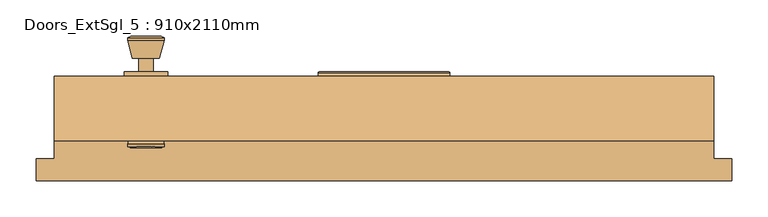
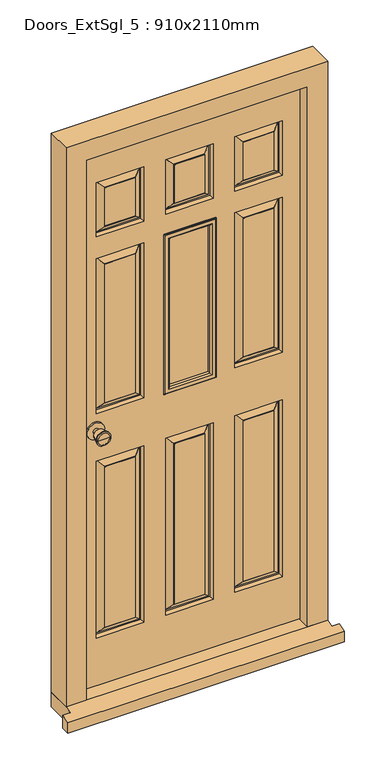
"""IFC4 building model written with IfcOpenShell, lengths in millimetres: door geometry, Doors_ExtSgl_5 : 910x2110mm."""

from ifc_helpers import new_model, si_unit, point, frame, frame_2d, origin, place, context, project, spatial, polyline, circle_curve, ellipse_curve, trimmed, segment, composite_curve, outline, extrude, faceted_brep, source, transform, mapped, element, save
from ifc_brep_helpers import plane_surface, cylinder_surface, revolved_surface, advanced_brep


def doors_extsgl_5_910x2110mm_99758a98(model_context):
    return source(origin(), model_context, "Body", "SolidModel", [
        advanced_brep(
        [(-328.4666667, 18.4, 1000.0), (-338.4666667, 18.4, 1000.0), (-318.4666667, 18.4, 1000.0), (-307.9907991, 67.4, 1000.0), (-348.9425342, 67.4, 1000.0), (-328.4666667, 67.4, 1000.0), (-303.4666667, 65.5721319, 1000.0), (-353.4666667, 65.5721319, 1000.0), (-303.4666667, 62.1084537, 1000.0), (-353.4666667, 62.1084537, 1000.0), (-309.8304306, 37.4, 1000.0), (-347.1029027, 37.4, 1000.0), (-318.4666667, 37.4, 1000.0), (-338.4666667, 37.4, 1000.0)],
        [
            (0, 1),
            (1, 2, circle_curve(frame((-328.4666667, 18.4, 1000.0), z_axis=(0.0, -1.0, 0.0), x_axis=(-1.0, 0.0, 0.0)), 10.0)),
            (2, 0),
            (2, 1, circle_curve(frame((-328.4666667, 18.4, 1000.0), z_axis=(0.0, -1.0, 0.0), x_axis=(-1.0, 0.0, 0.0)), 10.0)),
            (3, 4, circle_curve(frame((-328.4666667, 67.4, 1000.0), z_axis=(0.0, 1.0, 0.0), x_axis=(-1.0, 0.0, 0.0)), 20.4758676)),
            (4, 5),
            (5, 3),
            (4, 3, circle_curve(frame((-328.4666667, 67.4, 1000.0), z_axis=(0.0, 1.0, 0.0), x_axis=(-1.0, 0.0, 0.0)), 20.4758676)),
            (6, 7, circle_curve(frame((-328.4666667, 65.5721319, 1000.0), z_axis=(0.0, 1.0, 0.0), x_axis=(-1.0, 0.0, 0.0)), 25.0)),
            (7, 4),
            (3, 6),
            (7, 6, circle_curve(frame((-328.4666667, 65.5721319, 1000.0), z_axis=(0.0, 1.0, 0.0), x_axis=(-1.0, 0.0, 0.0)), 25.0)),
            (8, 9, circle_curve(frame((-328.4666667, 62.1084537, 1000.0), z_axis=(0.0, 1.0, 0.0), x_axis=(-1.0, 0.0, 0.0)), 25.0)),
            (9, 7),
            (6, 8),
            (9, 8, circle_curve(frame((-328.4666667, 62.1084537, 1000.0), z_axis=(0.0, 1.0, 0.0), x_axis=(-1.0, 0.0, 0.0)), 25.0)),
            (10, 11, circle_curve(frame((-328.4666667, 37.4, 1000.0), z_axis=(0.0, 1.0, 0.0), x_axis=(-1.0, 0.0, 0.0)), 18.636236)),
            (11, 9),
            (8, 10),
            (11, 10, circle_curve(frame((-328.4666667, 37.4, 1000.0), z_axis=(0.0, 1.0, 0.0), x_axis=(-1.0, 0.0, 0.0)), 18.636236)),
            (12, 13, circle_curve(frame((-328.4666667, 37.4, 1000.0), z_axis=(0.0, 1.0, 0.0), x_axis=(-1.0, 0.0, 0.0)), 10.0)),
            (13, 11),
            (10, 12),
            (13, 12, circle_curve(frame((-328.4666667, 37.4, 1000.0), z_axis=(0.0, 1.0, 0.0), x_axis=(-1.0, 0.0, 0.0)), 10.0)),
            (1, 13),
            (12, 2),
        ],
        [
            plane_surface(frame((-328.4666667, 18.4, 1000.0), z_axis=(0.0, -1.0, 0.0), x_axis=(-1.0, 0.0, 0.0))),
            plane_surface(frame((-328.4666667, 67.4, 1000.0), z_axis=(0.0, 1.0, 0.0), x_axis=(-1.0, 0.0, 0.0))),
            revolved_surface(polyline([(-348.9425342, 67.4, 1000.0), (-353.4666667, 65.5721319, 1000.0)]), (-328.4666667, 18.4, 1000.0), (0.0, -1.0, 0.0)),
            cylinder_surface(frame((-328.4666667, 18.4, 1000.0), z_axis=(0.0, -1.0, 0.0), x_axis=(-1.0, 0.0, 0.0)), 25.0),
            revolved_surface(polyline([(-353.4666667, 62.1084537, 1000.0), (-347.1029027, 37.4, 1000.0)]), (-328.4666667, 18.4, 1000.0), (0.0, -1.0, 0.0)),
            plane_surface(frame((-328.4666667, 37.4, 1000.0), z_axis=(0.0, -1.0, 0.0), x_axis=(-1.0, 0.0, 0.0))),
            cylinder_surface(frame((-328.4666667, 18.4, 1000.0), z_axis=(0.0, -1.0, 0.0), x_axis=(-1.0, 0.0, 0.0)), 10.0),
        ],
        [
            (0, [[1, 2, 3]]),
            (0, [[-3, 4, -1]]),
            (1, [[5, 6, 7]]),
            (1, [[8, -7, -6]]),
            (2, [[9, 10, -5, 11]]),
            (2, [[12, -11, -8, -10]]),
            (3, [[13, 14, -9, 15]]),
            (3, [[16, -15, -12, -14]]),
            (4, [[17, 18, -13, 19]]),
            (4, [[20, -19, -16, -18]]),
            (5, [[21, 22, -17, 23]]),
            (5, [[24, -23, -20, -22]]),
            (6, [[-2, 25, -21, 26]]),
            (6, [[-4, -26, -24, -25]]),
        ],
    ),
        extrude(outline(composite_curve([segment(trimmed(circle_curve(frame_2d((1000.0, -328.4666667)), 30.0), [point((1000.0, -358.4666667))], [point((1000.0, -298.4666667))], False, "CARTESIAN"), True, "CONTINUOUS"), segment(trimmed(circle_curve(frame_2d((1000.0, -328.4666667)), 30.0), [point((1000.0, -298.4666667))], [point((1000.0, -358.4666667))], False, "CARTESIAN"), True, "CONTINUOUS")], self_intersect=False)), frame((0.0, 12.4, 0.0), z_axis=(0.0, 1.0, 0.0), x_axis=(0.0, 0.0, 1.0)), (0.0, 0.0, 1.0), 6.0),
        advanced_brep(
        [(-328.4666667, -37.6, 1000.0), (-318.4666667, -37.6, 1000.0), (-338.4666667, -37.6, 1000.0), (-307.9907991, -86.6, 1000.0), (-328.4666667, -86.6, 1000.0), (-348.9425342, -86.6, 1000.0), (-303.4666667, -84.7721319, 1000.0), (-353.4666667, -84.7721319, 1000.0), (-303.4666667, -81.3084537, 1000.0), (-353.4666667, -81.3084537, 1000.0), (-309.8304306, -56.6, 1000.0), (-347.1029027, -56.6, 1000.0), (-318.4666667, -56.6, 1000.0), (-338.4666667, -56.6, 1000.0)],
        [
            (0, 1),
            (1, 2, circle_curve(frame((-328.4666667, -37.6, 1000.0), z_axis=(0.0, 1.0, 0.0), x_axis=(-1.0, 0.0, 0.0)), 10.0)),
            (2, 0),
            (2, 1, circle_curve(frame((-328.4666667, -37.6, 1000.0), z_axis=(0.0, 1.0, 0.0), x_axis=(-1.0, 0.0, 0.0)), 10.0)),
            (3, 4),
            (4, 5),
            (5, 3, circle_curve(frame((-328.4666667, -86.6, 1000.0), z_axis=(0.0, -1.0, 0.0), x_axis=(-1.0, 0.0, 0.0)), 20.4758676)),
            (3, 5, circle_curve(frame((-328.4666667, -86.6, 1000.0), z_axis=(0.0, -1.0, 0.0), x_axis=(-1.0, 0.0, 0.0)), 20.4758676)),
            (6, 3),
            (5, 7),
            (7, 6, circle_curve(frame((-328.4666667, -84.7721319, 1000.0), z_axis=(0.0, -1.0, 0.0), x_axis=(-1.0, 0.0, 0.0)), 25.0)),
            (6, 7, circle_curve(frame((-328.4666667, -84.7721319, 1000.0), z_axis=(0.0, -1.0, 0.0), x_axis=(-1.0, 0.0, 0.0)), 25.0)),
            (8, 6),
            (7, 9),
            (9, 8, circle_curve(frame((-328.4666667, -81.3084537, 1000.0), z_axis=(0.0, -1.0, 0.0), x_axis=(-1.0, 0.0, 0.0)), 25.0)),
            (8, 9, circle_curve(frame((-328.4666667, -81.3084537, 1000.0), z_axis=(0.0, -1.0, 0.0), x_axis=(-1.0, 0.0, 0.0)), 25.0)),
            (10, 8),
            (9, 11),
            (11, 10, circle_curve(frame((-328.4666667, -56.6, 1000.0), z_axis=(0.0, -1.0, 0.0), x_axis=(-1.0, 0.0, 0.0)), 18.636236)),
            (10, 11, circle_curve(frame((-328.4666667, -56.6, 1000.0), z_axis=(0.0, -1.0, 0.0), x_axis=(-1.0, 0.0, 0.0)), 18.636236)),
            (12, 10),
            (11, 13),
            (13, 12, circle_curve(frame((-328.4666667, -56.6, 1000.0), z_axis=(0.0, -1.0, 0.0), x_axis=(-1.0, 0.0, 0.0)), 10.0)),
            (12, 13, circle_curve(frame((-328.4666667, -56.6, 1000.0), z_axis=(0.0, -1.0, 0.0), x_axis=(-1.0, 0.0, 0.0)), 10.0)),
            (1, 12),
            (13, 2),
        ],
        [
            plane_surface(frame((-328.4666667, -37.6, 1000.0), z_axis=(0.0, 1.0, 0.0), x_axis=(-1.0, 0.0, 0.0))),
            plane_surface(frame((-328.4666667, -86.6, 1000.0), z_axis=(0.0, -1.0, 0.0), x_axis=(-1.0, 0.0, 0.0))),
            revolved_surface(polyline([(-348.9425342, -86.6, 1000.0), (-353.4666667, -84.7721319, 1000.0)]), (-328.4666667, -37.6, 1000.0), (0.0, 1.0, 0.0)),
            cylinder_surface(frame((-328.4666667, -37.6, 1000.0), z_axis=(0.0, 1.0, 0.0), x_axis=(-1.0, 0.0, 0.0)), 25.0),
            revolved_surface(polyline([(-353.4666667, -81.3084537, 1000.0), (-347.1029027, -56.6, 1000.0)]), (-328.4666667, -37.6, 1000.0), (0.0, 1.0, 0.0)),
            plane_surface(frame((-328.4666667, -56.6, 1000.0), z_axis=(0.0, 1.0, 0.0), x_axis=(-1.0, 0.0, 0.0))),
            cylinder_surface(frame((-328.4666667, -37.6, 1000.0), z_axis=(0.0, 1.0, 0.0), x_axis=(-1.0, 0.0, 0.0)), 10.0),
        ],
        [
            (0, [[1, 2, 3]]),
            (0, [[-3, 4, -1]]),
            (1, [[5, 6, 7]]),
            (1, [[-6, -5, 8]]),
            (2, [[9, -7, 10, 11]]),
            (2, [[-10, -8, -9, 12]]),
            (3, [[13, -11, 14, 15]]),
            (3, [[-14, -12, -13, 16]]),
            (4, [[17, -15, 18, 19]]),
            (4, [[-18, -16, -17, 20]]),
            (5, [[21, -19, 22, 23]]),
            (5, [[-22, -20, -21, 24]]),
            (6, [[25, -23, 26, -2]]),
            (6, [[-26, -24, -25, -4]]),
        ],
    ),
        extrude(outline(composite_curve([segment(trimmed(circle_curve(frame_2d((1000.0, -328.4666667)), 30.0), [point((1000.0, -358.4666667))], [point((1000.0, -298.4666667))], False, "CARTESIAN"), True, "CONTINUOUS"), segment(trimmed(circle_curve(frame_2d((1000.0, -328.4666667)), 30.0), [point((1000.0, -298.4666667))], [point((1000.0, -358.4666667))], False, "CARTESIAN"), True, "CONTINUOUS")], self_intersect=False)), frame((0.0, -37.6, 0.0), z_axis=(0.0, 1.0, 0.0), x_axis=(0.0, 0.0, 1.0)), (0.0, 0.0, 1.0), 6.0),
        faceted_brep([(384.5333333, -76.6, 54.5), (384.5333333, -34.6, 54.5), (406.5333333, -34.6, 54.5), (406.5333333, 12.4, 54.5), (455.0333333, 12.4, 54.5), (455.0333333, -76.6, 54.5), (455.0333333, -76.6, 2110.0), (-454.9666667, -76.6, 2110.0), (-454.9666667, -76.6, 54.5), (-384.4666667, -76.6, 54.5), (-384.4666667, -76.6, 2039.5), (384.5333333, -76.6, 2039.5), (455.0333333, 12.4, 2110.0), (406.5333333, 12.4, 2061.5), (-406.4666667, 12.4, 2061.5), (-406.4666667, 12.4, 54.5), (-454.9666667, 12.4, 54.5), (-454.9666667, 12.4, 2110.0), (406.5333333, -34.6, 2061.5), (384.5333333, -34.6, 2039.5), (-384.4666667, -34.6, 2039.5), (-384.4666667, -34.6, 54.5), (-406.4666667, -34.6, 54.5), (-406.4666667, -34.6, 2061.5)], [[[0, 1, 2, 3, 4, 5]], [[5, 6, 7, 8, 9, 10, 11, 0]], [[4, 12, 6, 5]], [[3, 13, 14, 15, 16, 17, 12, 4]], [[2, 18, 13, 3]], [[1, 19, 20, 21, 22, 23, 18, 2]], [[0, 11, 19, 1]], [[9, 21, 20, 10]], [[8, 16, 15, 22, 21, 9]], [[7, 17, 16, 8]], [[14, 23, 22, 15]], [[6, 12, 17, 7]], [[13, 18, 23, 14]], [[10, 20, 19, 11]]]),
        faceted_brep([(403.5333333, 12.4, 58.5), (-404.3916961, 12.4, 58.5), (-404.3916961, 12.4, 2058.5), (403.5333333, 12.4, 2058.5), (-82.8, 12.4, 1058.5), (82.8666667, 12.4, 1058.5), (82.8666667, 12.4, 1628.5), (-82.8, 12.4, 1628.5), (-157.8, 12.4, 883.5), (-323.4666667, 12.4, 883.5), (-323.4666667, 12.4, 233.5), (-157.8, 12.4, 233.5), (323.5333333, 12.4, 883.5), (157.8666667, 12.4, 883.5), (157.8666667, 12.4, 233.5), (323.5333333, 12.4, 233.5), (82.8666667, 12.4, 883.5), (-82.8, 12.4, 883.5), (-82.8, 12.4, 233.5), (82.8666667, 12.4, 233.5), (-323.4666667, 12.4, 1058.5), (-157.8, 12.4, 1058.5), (-157.8, 12.4, 1628.5), (-323.4666667, 12.4, 1628.5), (323.5333333, 12.4, 1628.5), (157.8666667, 12.4, 1628.5), (157.8666667, 12.4, 1058.5), (323.5333333, 12.4, 1058.5), (-157.8, 12.4, 1908.5), (-323.4666667, 12.4, 1908.5), (-323.4666667, 12.4, 1708.5), (-157.8, 12.4, 1708.5), (82.8666667, 12.4, 1908.5), (-82.8, 12.4, 1908.5), (-82.8, 12.4, 1708.5), (82.8666667, 12.4, 1708.5), (323.5333333, 12.4, 1908.5), (157.8666667, 12.4, 1908.5), (157.8666667, 12.4, 1708.5), (323.5333333, 12.4, 1708.5), (-187.8, 12.4, 263.5), (-293.4666667, 12.4, 263.5), (-293.4666667, 12.4, 853.5), (-187.8, 12.4, 853.5), (293.5333333, 12.4, 263.5), (187.8666667, 12.4, 263.5), (187.8666667, 12.4, 853.5), (293.5333333, 12.4, 853.5), (52.8666667, 12.4, 263.5), (-52.8, 12.4, 263.5), (-52.8, 12.4, 853.5), (52.8666667, 12.4, 853.5), (-293.4666667, 12.4, 1598.5), (-187.8, 12.4, 1598.5), (-187.8, 12.4, 1088.5), (-293.4666667, 12.4, 1088.5), (293.5333333, 12.4, 1088.5), (187.8666667, 12.4, 1088.5), (187.8666667, 12.4, 1598.5), (293.5333333, 12.4, 1598.5), (-187.8, 12.4, 1738.5), (-293.4666667, 12.4, 1738.5), (-293.4666667, 12.4, 1878.5), (-187.8, 12.4, 1878.5), (52.8666667, 12.4, 1738.5), (-52.8, 12.4, 1738.5), (-52.8, 12.4, 1878.5), (52.8666667, 12.4, 1878.5), (293.5333333, 12.4, 1738.5), (187.8666667, 12.4, 1738.5), (187.8666667, 12.4, 1878.5), (293.5333333, 12.4, 1878.5), (403.5333333, -31.6, 58.5), (403.5333333, -31.6, 2058.5), (-404.3916961, -31.6, 2058.5), (-404.3916961, -31.6, 58.5), (-82.8, -31.6, 1058.5), (-82.8, -31.6, 1628.5), (82.8666667, -31.6, 1628.5), (82.8666667, -31.6, 1058.5), (157.8666667, -31.6, 883.5), (323.5333333, -31.6, 883.5), (323.5333333, -31.6, 233.5), (157.8666667, -31.6, 233.5), (-323.4666667, -31.6, 883.5), (-157.8, -31.6, 883.5), (-157.8, -31.6, 233.5), (-323.4666667, -31.6, 233.5), (-82.8, -31.6, 883.5), (82.8666667, -31.6, 883.5), (82.8666667, -31.6, 233.5), (-82.8, -31.6, 233.5), (157.8666667, -31.6, 1628.5), (323.5333333, -31.6, 1628.5), (323.5333333, -31.6, 1058.5), (157.8666667, -31.6, 1058.5), (-323.4666667, -31.6, 1628.5), (-157.8, -31.6, 1628.5), (-157.8, -31.6, 1058.5), (-323.4666667, -31.6, 1058.5), (323.5333333, -31.6, 1708.5), (157.8666667, -31.6, 1708.5), (157.8666667, -31.6, 1908.5), (323.5333333, -31.6, 1908.5), (-82.8, -31.6, 1908.5), (82.8666667, -31.6, 1908.5), (82.8666667, -31.6, 1708.5), (-82.8, -31.6, 1708.5), (-323.4666667, -31.6, 1908.5), (-157.8, -31.6, 1908.5), (-157.8, -31.6, 1708.5), (-323.4666667, -31.6, 1708.5), (187.8666667, -31.6, 263.5), (293.5333333, -31.6, 263.5), (293.5333333, -31.6, 853.5), (187.8666667, -31.6, 853.5), (-293.4666667, -31.6, 263.5), (-187.8, -31.6, 263.5), (-187.8, -31.6, 853.5), (-293.4666667, -31.6, 853.5), (-52.8, -31.6, 263.5), (52.8666667, -31.6, 263.5), (52.8666667, -31.6, 853.5), (-52.8, -31.6, 853.5), (187.8666667, -31.6, 1088.5), (293.5333333, -31.6, 1088.5), (293.5333333, -31.6, 1598.5), (187.8666667, -31.6, 1598.5), (-293.4666667, -31.6, 1088.5), (-187.8, -31.6, 1088.5), (-187.8, -31.6, 1598.5), (-293.4666667, -31.6, 1598.5), (293.5333333, -31.6, 1878.5), (187.8666667, -31.6, 1878.5), (187.8666667, -31.6, 1738.5), (293.5333333, -31.6, 1738.5), (-52.8, -31.6, 1738.5), (52.8666667, -31.6, 1738.5), (52.8666667, -31.6, 1878.5), (-52.8, -31.6, 1878.5), (-293.4666667, -31.6, 1738.5), (-187.8, -31.6, 1738.5), (-187.8, -31.6, 1878.5), (-293.4666667, -31.6, 1878.5), (160.8666667, -16.6, 880.5), (160.8666667, -16.6, 236.5), (185.8666667, -30.6, 855.5), (165.8666667, -16.6, 875.5), (165.8666667, -16.6, 241.5), (185.8666667, -30.6, 261.5), (187.8666667, -30.6, 853.5), (187.8666667, -30.6, 263.5), (320.5333333, -16.6, 236.5), (315.5333333, -16.6, 241.5), (295.5333333, -30.6, 261.5), (293.5333333, -30.6, 263.5), (320.5333333, -16.6, 880.5), (315.5333333, -16.6, 875.5), (295.5333333, -30.6, 855.5), (293.5333333, -30.6, 853.5), (-320.4666667, -16.6, 880.5), (-320.4666667, -16.6, 236.5), (-295.4666667, -30.6, 855.5), (-315.4666667, -16.6, 875.5), (-315.4666667, -16.6, 241.5), (-295.4666667, -30.6, 261.5), (-293.4666667, -30.6, 853.5), (-293.4666667, -30.6, 263.5), (-160.8, -16.6, 236.5), (-165.8, -16.6, 241.5), (-185.8, -30.6, 261.5), (-187.8, -30.6, 263.5), (-160.8, -16.6, 880.5), (-165.8, -16.6, 875.5), (-185.8, -30.6, 855.5), (-187.8, -30.6, 853.5), (-187.8, 11.4, 263.5), (-187.8, 11.4, 853.5), (-165.8, -2.6, 241.5), (-185.8, 11.4, 261.5), (-185.8, 11.4, 855.5), (-165.8, -2.6, 875.5), (-160.8, -2.6, 236.5), (-160.8, -2.6, 880.5), (-293.4666667, 11.4, 853.5), (-295.4666667, 11.4, 855.5), (-315.4666667, -2.6, 875.5), (-320.4666667, -2.6, 880.5), (-293.4666667, 11.4, 263.5), (-295.4666667, 11.4, 261.5), (-315.4666667, -2.6, 241.5), (-320.4666667, -2.6, 236.5), (320.5333333, -2.6, 880.5), (320.5333333, -2.6, 236.5), (295.5333333, 11.4, 855.5), (315.5333333, -2.6, 875.5), (315.5333333, -2.6, 241.5), (295.5333333, 11.4, 261.5), (293.5333333, 11.4, 853.5), (293.5333333, 11.4, 263.5), (160.8666667, -2.6, 236.5), (165.8666667, -2.6, 241.5), (185.8666667, 11.4, 261.5), (187.8666667, 11.4, 263.5), (160.8666667, -2.6, 880.5), (165.8666667, -2.6, 875.5), (185.8666667, 11.4, 855.5), (187.8666667, 11.4, 853.5), (-52.8, -30.6, 263.5), (-52.8, -30.6, 853.5), (-74.8, -16.6, 241.5), (-54.8, -30.6, 261.5), (-54.8, -30.6, 855.5), (-74.8, -16.6, 875.5), (-79.8, -16.6, 236.5), (-79.8, -16.6, 880.5), (52.8666667, -30.6, 853.5), (54.8666667, -30.6, 855.5), (74.8666667, -16.6, 875.5), (79.8666667, -16.6, 880.5), (52.8666667, -30.6, 263.5), (54.8666667, -30.6, 261.5), (74.8666667, -16.6, 241.5), (79.8666667, -16.6, 236.5), (79.8666667, -2.6, 880.5), (79.8666667, -2.6, 236.5), (54.8666667, 11.4, 855.5), (74.8666667, -2.6, 875.5), (74.8666667, -2.6, 241.5), (54.8666667, 11.4, 261.5), (52.8666667, 11.4, 853.5), (52.8666667, 11.4, 263.5), (-79.8, -2.6, 236.5), (-74.8, -2.6, 241.5), (-54.8, 11.4, 261.5), (-52.8, 11.4, 263.5), (-79.8, -2.6, 880.5), (-74.8, -2.6, 875.5), (-54.8, 11.4, 855.5), (-52.8, 11.4, 853.5), (187.8666667, -30.6, 1088.5), (187.8666667, -30.6, 1598.5), (165.8666667, -16.6, 1066.5), (185.8666667, -30.6, 1086.5), (185.8666667, -30.6, 1600.5), (165.8666667, -16.6, 1620.5), (160.8666667, -16.6, 1061.5), (160.8666667, -16.6, 1625.5), (293.5333333, -30.6, 1598.5), (295.5333333, -30.6, 1600.5), (315.5333333, -16.6, 1620.5), (320.5333333, -16.6, 1625.5), (293.5333333, -30.6, 1088.5), (295.5333333, -30.6, 1086.5), (315.5333333, -16.6, 1066.5), (320.5333333, -16.6, 1061.5), (-293.4666667, -30.6, 1088.5), (-293.4666667, -30.6, 1598.5), (-315.4666667, -16.6, 1066.5), (-295.4666667, -30.6, 1086.5), (-295.4666667, -30.6, 1600.5), (-315.4666667, -16.6, 1620.5), (-320.4666667, -16.6, 1061.5), (-320.4666667, -16.6, 1625.5), (-187.8, -30.6, 1598.5), (-185.8, -30.6, 1600.5), (-165.8, -16.6, 1620.5), (-160.8, -16.6, 1625.5), (-187.8, -30.6, 1088.5), (-185.8, -30.6, 1086.5), (-165.8, -16.6, 1066.5), (-160.8, -16.6, 1061.5), (293.5333333, -30.6, 1878.5), (293.5333333, -30.6, 1738.5), (315.5333333, -16.6, 1900.5), (295.5333333, -30.6, 1880.5), (295.5333333, -30.6, 1736.5), (315.5333333, -16.6, 1716.5), (320.5333333, -16.6, 1905.5), (320.5333333, -16.6, 1711.5), (187.8666667, -30.6, 1738.5), (185.8666667, -30.6, 1736.5), (165.8666667, -16.6, 1716.5), (160.8666667, -16.6, 1711.5), (187.8666667, -30.6, 1878.5), (185.8666667, -30.6, 1880.5), (165.8666667, -16.6, 1900.5), (160.8666667, -16.6, 1905.5), (-52.8, -30.6, 1738.5), (-52.8, -30.6, 1878.5), (-74.8, -16.6, 1716.5), (-54.8, -30.6, 1736.5), (-54.8, -30.6, 1880.5), (-74.8, -16.6, 1900.5), (-79.8, -16.6, 1711.5), (-79.8, -16.6, 1905.5), (52.8666667, -30.6, 1878.5), (54.8666667, -30.6, 1880.5), (74.8666667, -16.6, 1900.5), (79.8666667, -16.6, 1905.5), (52.8666667, -30.6, 1738.5), (54.8666667, -30.6, 1736.5), (74.8666667, -16.6, 1716.5), (79.8666667, -16.6, 1711.5), (-293.4666667, -30.6, 1738.5), (-293.4666667, -30.6, 1878.5), (-315.4666667, -16.6, 1716.5), (-295.4666667, -30.6, 1736.5), (-295.4666667, -30.6, 1880.5), (-315.4666667, -16.6, 1900.5), (-320.4666667, -16.6, 1711.5), (-320.4666667, -16.6, 1905.5), (-187.8, -30.6, 1878.5), (-185.8, -30.6, 1880.5), (-165.8, -16.6, 1900.5), (-160.8, -16.6, 1905.5), (-187.8, -30.6, 1738.5), (-185.8, -30.6, 1736.5), (-165.8, -16.6, 1716.5), (-160.8, -16.6, 1711.5), (-320.4666667, -2.6, 1061.5), (-320.4666667, -2.6, 1625.5), (-295.4666667, 11.4, 1086.5), (-315.4666667, -2.6, 1066.5), (-315.4666667, -2.6, 1620.5), (-295.4666667, 11.4, 1600.5), (-293.4666667, 11.4, 1088.5), (-293.4666667, 11.4, 1598.5), (-160.8, -2.6, 1625.5), (-165.8, -2.6, 1620.5), (-185.8, 11.4, 1600.5), (-187.8, 11.4, 1598.5), (-160.8, -2.6, 1061.5), (-165.8, -2.6, 1066.5), (-185.8, 11.4, 1086.5), (-187.8, 11.4, 1088.5), (320.5333333, -2.6, 1625.5), (320.5333333, -2.6, 1061.5), (295.5333333, 11.4, 1600.5), (315.5333333, -2.6, 1620.5), (315.5333333, -2.6, 1066.5), (295.5333333, 11.4, 1086.5), (293.5333333, 11.4, 1598.5), (293.5333333, 11.4, 1088.5), (160.8666667, -2.6, 1061.5), (165.8666667, -2.6, 1066.5), (185.8666667, 11.4, 1086.5), (187.8666667, 11.4, 1088.5), (160.8666667, -2.6, 1625.5), (165.8666667, -2.6, 1620.5), (185.8666667, 11.4, 1600.5), (187.8666667, 11.4, 1598.5), (-187.8, 11.4, 1738.5), (-187.8, 11.4, 1878.5), (-165.8, -2.6, 1716.5), (-185.8, 11.4, 1736.5), (-185.8, 11.4, 1880.5), (-165.8, -2.6, 1900.5), (-160.8, -2.6, 1711.5), (-160.8, -2.6, 1905.5), (-293.4666667, 11.4, 1878.5), (-295.4666667, 11.4, 1880.5), (-315.4666667, -2.6, 1900.5), (-320.4666667, -2.6, 1905.5), (-293.4666667, 11.4, 1738.5), (-295.4666667, 11.4, 1736.5), (-315.4666667, -2.6, 1716.5), (-320.4666667, -2.6, 1711.5), (52.8666667, 11.4, 1738.5), (52.8666667, 11.4, 1878.5), (74.8666667, -2.6, 1716.5), (54.8666667, 11.4, 1736.5), (54.8666667, 11.4, 1880.5), (74.8666667, -2.6, 1900.5), (79.8666667, -2.6, 1711.5), (79.8666667, -2.6, 1905.5), (-52.8, 11.4, 1878.5), (-54.8, 11.4, 1880.5), (-74.8, -2.6, 1900.5), (-79.8, -2.6, 1905.5), (-52.8, 11.4, 1738.5), (-54.8, 11.4, 1736.5), (-74.8, -2.6, 1716.5), (-79.8, -2.6, 1711.5), (293.5333333, 11.4, 1738.5), (293.5333333, 11.4, 1878.5), (315.5333333, -2.6, 1716.5), (295.5333333, 11.4, 1736.5), (295.5333333, 11.4, 1880.5), (315.5333333, -2.6, 1900.5), (320.5333333, -2.6, 1711.5), (320.5333333, -2.6, 1905.5), (187.8666667, 11.4, 1878.5), (185.8666667, 11.4, 1880.5), (165.8666667, -2.6, 1900.5), (160.8666667, -2.6, 1905.5), (187.8666667, 11.4, 1738.5), (185.8666667, 11.4, 1736.5), (165.8666667, -2.6, 1716.5), (160.8666667, -2.6, 1711.5)], [[[0, 1, 2, 3], [4, 5, 6, 7], [8, 9, 10, 11], [12, 13, 14, 15], [16, 17, 18, 19], [20, 21, 22, 23], [24, 25, 26, 27], [28, 29, 30, 31], [32, 33, 34, 35], [36, 37, 38, 39]], [[40, 41, 42, 43]], [[44, 45, 46, 47]], [[48, 49, 50, 51]], [[52, 53, 54, 55]], [[56, 57, 58, 59]], [[60, 61, 62, 63]], [[64, 65, 66, 67]], [[68, 69, 70, 71]], [[72, 73, 74, 75], [76, 77, 78, 79], [80, 81, 82, 83], [84, 85, 86, 87], [88, 89, 90, 91], [92, 93, 94, 95], [96, 97, 98, 99], [100, 101, 102, 103], [104, 105, 106, 107], [108, 109, 110, 111]], [[112, 113, 114, 115]], [[116, 117, 118, 119]], [[120, 121, 122, 123]], [[124, 125, 126, 127]], [[128, 129, 130, 131]], [[132, 133, 134, 135]], [[136, 137, 138, 139]], [[140, 141, 142, 143]], [[3, 73, 72, 0]], [[2, 74, 73, 3]], [[1, 75, 74, 2]], [[0, 72, 75, 1]], [[7, 77, 76, 4]], [[6, 78, 77, 7]], [[5, 79, 78, 6]], [[4, 76, 79, 5]], [[144, 80, 83, 145]], [[146, 147, 148, 149]], [[112, 115, 150, 151]], [[83, 82, 152, 145]], [[148, 153, 154, 149]], [[151, 155, 113, 112]], [[82, 81, 156, 152]], [[153, 157, 158, 154]], [[155, 159, 114, 113]], [[144, 156, 81, 80]], [[145, 152, 156, 144], [147, 157, 153, 148]], [[146, 158, 157, 147]], [[149, 154, 158, 146], [150, 159, 155, 151]], [[115, 114, 159, 150]], [[160, 84, 87, 161]], [[162, 163, 164, 165]], [[116, 119, 166, 167]], [[87, 86, 168, 161]], [[164, 169, 170, 165]], [[167, 171, 117, 116]], [[86, 85, 172, 168]], [[169, 173, 174, 170]], [[171, 175, 118, 117]], [[160, 172, 85, 84]], [[161, 168, 172, 160], [163, 173, 169, 164]], [[162, 174, 173, 163]], [[165, 170, 174, 162], [166, 175, 171, 167]], [[119, 118, 175, 166]], [[176, 40, 43, 177]], [[178, 179, 180, 181]], [[8, 11, 182, 183]], [[43, 42, 184, 177]], [[180, 185, 186, 181]], [[183, 187, 9, 8]], [[42, 41, 188, 184]], [[185, 189, 190, 186]], [[187, 191, 10, 9]], [[176, 188, 41, 40]], [[179, 189, 185, 180], [177, 184, 188, 176]], [[178, 190, 189, 179]], [[182, 191, 187, 183], [181, 186, 190, 178]], [[11, 10, 191, 182]], [[192, 12, 15, 193]], [[194, 195, 196, 197]], [[44, 47, 198, 199]], [[15, 14, 200, 193]], [[196, 201, 202, 197]], [[199, 203, 45, 44]], [[14, 13, 204, 200]], [[201, 205, 206, 202]], [[203, 207, 46, 45]], [[192, 204, 13, 12]], [[193, 200, 204, 192], [195, 205, 201, 196]], [[194, 206, 205, 195]], [[197, 202, 206, 194], [198, 207, 203, 199]], [[47, 46, 207, 198]], [[208, 120, 123, 209]], [[210, 211, 212, 213]], [[88, 91, 214, 215]], [[123, 122, 216, 209]], [[212, 217, 218, 213]], [[215, 219, 89, 88]], [[122, 121, 220, 216]], [[217, 221, 222, 218]], [[219, 223, 90, 89]], [[208, 220, 121, 120]], [[211, 221, 217, 212], [209, 216, 220, 208]], [[210, 222, 221, 211]], [[214, 223, 219, 215], [213, 218, 222, 210]], [[91, 90, 223, 214]], [[224, 16, 19, 225]], [[226, 227, 228, 229]], [[48, 51, 230, 231]], [[19, 18, 232, 225]], [[228, 233, 234, 229]], [[231, 235, 49, 48]], [[18, 17, 236, 232]], [[233, 237, 238, 234]], [[235, 239, 50, 49]], [[224, 236, 17, 16]], [[225, 232, 236, 224], [227, 237, 233, 228]], [[226, 238, 237, 227]], [[229, 234, 238, 226], [230, 239, 235, 231]], [[51, 50, 239, 230]], [[240, 124, 127, 241]], [[242, 243, 244, 245]], [[92, 95, 246, 247]], [[127, 126, 248, 241]], [[244, 249, 250, 245]], [[247, 251, 93, 92]], [[126, 125, 252, 248]], [[249, 253, 254, 250]], [[251, 255, 94, 93]], [[240, 252, 125, 124]], [[243, 253, 249, 244], [241, 248, 252, 240]], [[242, 254, 253, 243]], [[246, 255, 251, 247], [245, 250, 254, 242]], [[95, 94, 255, 246]], [[256, 128, 131, 257]], [[258, 259, 260, 261]], [[96, 99, 262, 263]], [[131, 130, 264, 257]], [[260, 265, 266, 261]], [[263, 267, 97, 96]], [[130, 129, 268, 264]], [[265, 269, 270, 266]], [[267, 271, 98, 97]], [[256, 268, 129, 128]], [[259, 269, 265, 260], [257, 264, 268, 256]], [[258, 270, 269, 259]], [[262, 271, 267, 263], [261, 266, 270, 258]], [[99, 98, 271, 262]], [[272, 132, 135, 273]], [[274, 275, 276, 277]], [[100, 103, 278, 279]], [[135, 134, 280, 273]], [[276, 281, 282, 277]], [[279, 283, 101, 100]], [[134, 133, 284, 280]], [[281, 285, 286, 282]], [[283, 287, 102, 101]], [[272, 284, 133, 132]], [[275, 285, 281, 276], [273, 280, 284, 272]], [[274, 286, 285, 275]], [[278, 287, 283, 279], [277, 282, 286, 274]], [[103, 102, 287, 278]], [[288, 136, 139, 289]], [[290, 291, 292, 293]], [[104, 107, 294, 295]], [[139, 138, 296, 289]], [[292, 297, 298, 293]], [[295, 299, 105, 104]], [[138, 137, 300, 296]], [[297, 301, 302, 298]], [[299, 303, 106, 105]], [[288, 300, 137, 136]], [[291, 301, 297, 292], [289, 296, 300, 288]], [[290, 302, 301, 291]], [[294, 303, 299, 295], [293, 298, 302, 290]], [[107, 106, 303, 294]], [[304, 140, 143, 305]], [[306, 307, 308, 309]], [[108, 111, 310, 311]], [[143, 142, 312, 305]], [[308, 313, 314, 309]], [[311, 315, 109, 108]], [[142, 141, 316, 312]], [[313, 317, 318, 314]], [[315, 319, 110, 109]], [[304, 316, 141, 140]], [[307, 317, 313, 308], [305, 312, 316, 304]], [[306, 318, 317, 307]], [[310, 319, 315, 311], [309, 314, 318, 306]], [[111, 110, 319, 310]], [[320, 20, 23, 321]], [[322, 323, 324, 325]], [[52, 55, 326, 327]], [[23, 22, 328, 321]], [[324, 329, 330, 325]], [[327, 331, 53, 52]], [[22, 21, 332, 328]], [[329, 333, 334, 330]], [[331, 335, 54, 53]], [[320, 332, 21, 20]], [[321, 328, 332, 320], [323, 333, 329, 324]], [[322, 334, 333, 323]], [[325, 330, 334, 322], [326, 335, 331, 327]], [[55, 54, 335, 326]], [[336, 24, 27, 337]], [[338, 339, 340, 341]], [[56, 59, 342, 343]], [[27, 26, 344, 337]], [[340, 345, 346, 341]], [[343, 347, 57, 56]], [[26, 25, 348, 344]], [[345, 349, 350, 346]], [[347, 351, 58, 57]], [[336, 348, 25, 24]], [[337, 344, 348, 336], [339, 349, 345, 340]], [[338, 350, 349, 339]], [[341, 346, 350, 338], [342, 351, 347, 343]], [[59, 58, 351, 342]], [[352, 60, 63, 353]], [[354, 355, 356, 357]], [[28, 31, 358, 359]], [[63, 62, 360, 353]], [[356, 361, 362, 357]], [[359, 363, 29, 28]], [[62, 61, 364, 360]], [[361, 365, 366, 362]], [[363, 367, 30, 29]], [[352, 364, 61, 60]], [[355, 365, 361, 356], [353, 360, 364, 352]], [[354, 366, 365, 355]], [[358, 367, 363, 359], [357, 362, 366, 354]], [[31, 30, 367, 358]], [[368, 64, 67, 369]], [[370, 371, 372, 373]], [[32, 35, 374, 375]], [[67, 66, 376, 369]], [[372, 377, 378, 373]], [[375, 379, 33, 32]], [[66, 65, 380, 376]], [[377, 381, 382, 378]], [[379, 383, 34, 33]], [[368, 380, 65, 64]], [[371, 381, 377, 372], [369, 376, 380, 368]], [[370, 382, 381, 371]], [[374, 383, 379, 375], [373, 378, 382, 370]], [[35, 34, 383, 374]], [[384, 68, 71, 385]], [[386, 387, 388, 389]], [[36, 39, 390, 391]], [[71, 70, 392, 385]], [[388, 393, 394, 389]], [[391, 395, 37, 36]], [[70, 69, 396, 392]], [[393, 397, 398, 394]], [[395, 399, 38, 37]], [[384, 396, 69, 68]], [[387, 397, 393, 388], [385, 392, 396, 384]], [[386, 398, 397, 387]], [[390, 399, 395, 391], [389, 394, 398, 386]], [[39, 38, 399, 390]]]),
        faceted_brep([(480.0333333, -131.6, 0.0), (480.0333333, -101.6, 0.0), (480.0333333, -101.6, 47.2703282), (480.0333333, -131.6, 38.5947221), (-479.9666667, -131.6, 38.5947221), (-479.9666667, -101.6, 47.2703282), (-479.9666667, -101.6, 0.0), (-479.9666667, -131.6, 0.0), (-454.9666667, -101.6, 0.0), (-454.9666667, 12.4, 0.0), (455.0333333, 12.4, 0.0), (455.0333333, -101.6, 0.0), (455.0333333, -101.6, 47.2703282), (455.0333333, -76.6, 54.5), (-454.9666667, -76.6, 54.5), (-454.9666667, -101.6, 47.2703282), (455.0333333, 12.4, 54.5), (-454.9666667, 12.4, 54.5)], [[[0, 1, 2, 3]], [[4, 5, 6, 7]], [[7, 6, 8, 9, 10, 11, 1, 0]], [[3, 4, 7, 0]], [[3, 2, 12, 13, 14, 15, 5, 4]], [[14, 13, 16, 17]], [[17, 16, 10, 9]], [[15, 14, 17, 9, 8]], [[8, 6, 5, 15]], [[11, 10, 16, 13, 12]], [[12, 2, 1, 11]]]),
        extrude(outline(polyline([(82.8666667, 2.4), (82.8666667, -21.6), (-82.8, -21.6), (-82.8, 2.4), (82.8666667, 2.4)])), frame((0.0, 0.0, 1058.5), z_axis=(0.0, 0.0, 1.0), x_axis=(1.0, 0.0, 0.0)), (0.0, 0.0, 1.0), 570.0),
        advanced_brep(
        [(-90.8, -35.6, 1050.5), (-90.8, -35.6, 1636.5), (-90.8, -31.6, 1636.5), (-90.8, -31.6, 1050.5), (-88.8, -37.6, 1052.5), (-88.8, -37.6, 1634.5), (-70.8, -32.6, 1070.5), (-70.8, -32.6, 1616.5), (-75.8, -37.6, 1621.5), (-75.8, -37.6, 1065.5), (-70.8, -21.6, 1070.5), (-70.8, -21.6, 1616.5), (-82.8, -31.6, 1058.5), (-82.8, -31.6, 1628.5), (-82.8, -21.6, 1628.5), (-82.8, -21.6, 1058.5), (90.8666667, -35.6, 1636.5), (90.8666667, -31.6, 1636.5), (88.8666667, -37.6, 1634.5), (70.8666667, -32.6, 1616.5), (75.8666667, -37.6, 1621.5), (70.8666667, -21.6, 1616.5), (82.8666667, -31.6, 1628.5), (82.8666667, -21.6, 1628.5), (90.8666667, -35.6, 1050.5), (90.8666667, -31.6, 1050.5), (88.8666667, -37.6, 1052.5), (70.8666667, -32.6, 1070.5), (75.8666667, -37.6, 1065.5), (70.8666667, -21.6, 1070.5), (82.8666667, -31.6, 1058.5), (82.8666667, -21.6, 1058.5)],
        [
            (0, 1),
            (1, 2),
            (2, 3),
            (3, 0),
            (4, 5),
            (5, 1, ellipse_curve(frame((-88.8, -35.6, 1634.5), z_axis=(-0.7071067811865475, 0.0, -0.7071067811865475), x_axis=(0.7071067811865474, 0.0, -0.7071067811865476)), 2.8284271, 2.0)),
            (0, 4, ellipse_curve(frame((-88.8, -35.6, 1052.5), z_axis=(-0.7071067811865475, 0.0, 0.7071067811865475), x_axis=(-0.7071067811865474, 0.0, -0.7071067811865476)), 2.8284271, 2.0)),
            (6, 7),
            (7, 8, ellipse_curve(frame((-75.8, -32.6, 1621.5), z_axis=(-0.7071067811865475, 0.0, -0.7071067811865475), x_axis=(0.7071067811865474, 0.0, -0.7071067811865476)), 7.0710678, 5.0)),
            (8, 9),
            (9, 6, ellipse_curve(frame((-75.8, -32.6, 1065.5), z_axis=(-0.7071067811865475, 0.0, 0.7071067811865475), x_axis=(-0.7071067811865474, 0.0, -0.7071067811865476)), 7.0710678, 5.0)),
            (10, 11),
            (11, 7),
            (6, 10),
            (12, 13),
            (13, 14),
            (14, 15),
            (15, 12),
            (1, 16),
            (16, 17),
            (17, 2),
            (5, 18),
            (18, 16, ellipse_curve(frame((88.8666667, -35.6, 1634.5), z_axis=(-0.7071067811865475, 0.0, 0.7071067811865475), x_axis=(-0.7071067811865476, 0.0, -0.7071067811865474)), 2.8284271, 2.0)),
            (7, 19),
            (19, 20, ellipse_curve(frame((75.8666667, -32.6, 1621.5), z_axis=(-0.7071067811865475, 0.0, 0.7071067811865475), x_axis=(-0.7071067811865476, 0.0, -0.7071067811865474)), 7.0710678, 5.0)),
            (20, 8),
            (11, 21),
            (21, 19),
            (13, 22),
            (22, 23),
            (23, 14),
            (16, 24),
            (24, 25),
            (25, 17),
            (18, 26),
            (26, 24, ellipse_curve(frame((88.8666667, -35.6, 1052.5), z_axis=(0.7071067811865475, 0.0, 0.7071067811865475), x_axis=(-0.7071067811865474, 0.0, 0.7071067811865476)), 2.8284271, 2.0)),
            (19, 27),
            (27, 28, ellipse_curve(frame((75.8666667, -32.6, 1065.5), z_axis=(0.7071067811865475, 0.0, 0.7071067811865475), x_axis=(-0.7071067811865474, 0.0, 0.7071067811865476)), 7.0710678, 5.0)),
            (28, 20),
            (21, 29),
            (29, 27),
            (22, 30),
            (30, 31),
            (31, 23),
            (24, 0),
            (3, 25),
            (26, 4),
            (28, 9),
            (27, 6),
            (29, 10),
            (31, 15),
            (30, 12),
        ],
        [
            plane_surface(frame((-90.8, -31.6, 1050.5), z_axis=(-1.0, 0.0, 0.0), x_axis=(0.0, 0.0, 1.0))),
            cylinder_surface(frame((-88.8, -35.6, 1058.5), z_axis=(0.0, 0.0, -1.0), x_axis=(-1.0, 0.0, 0.0)), 2.0),
            cylinder_surface(frame((-75.8, -32.6, 1058.5), z_axis=(0.0, 0.0, -1.0), x_axis=(-1.0, 0.0, 0.0)), 5.0),
            plane_surface(frame((-70.8, -32.6, 1070.5), z_axis=(1.0, 0.0, 0.0), x_axis=(0.0, 0.0, 1.0))),
            plane_surface(frame((-82.8, -21.6, 1058.5), z_axis=(-1.0, 0.0, 0.0), x_axis=(0.0, 0.0, 1.0))),
            plane_surface(frame((-90.8, -31.6, 1636.5), z_axis=(0.0, 0.0, 1.0), x_axis=(1.0, 0.0, 0.0))),
            cylinder_surface(frame((-82.8, -35.6, 1634.5), z_axis=(-1.0, 0.0, 0.0), x_axis=(0.0, 0.0, 1.0)), 2.0),
            cylinder_surface(frame((-82.8, -32.6, 1621.5), z_axis=(-1.0, 0.0, 0.0), x_axis=(0.0, 0.0, 1.0)), 5.0),
            plane_surface(frame((-70.8, -32.6, 1616.5), z_axis=(0.0, 0.0, -1.0), x_axis=(1.0, 0.0, 0.0))),
            plane_surface(frame((-82.8, -21.6, 1628.5), z_axis=(0.0, 0.0, 1.0), x_axis=(1.0, 0.0, 0.0))),
            plane_surface(frame((90.8666667, -31.6, 1636.5), z_axis=(1.0, 0.0, 0.0), x_axis=(0.0, 0.0, -1.0))),
            cylinder_surface(frame((88.8666667, -35.6, 1628.5), z_axis=(0.0, 0.0, 1.0), x_axis=(1.0, 0.0, 0.0)), 2.0),
            cylinder_surface(frame((75.8666667, -32.6, 1628.5), z_axis=(0.0, 0.0, 1.0), x_axis=(1.0, 0.0, 0.0)), 5.0),
            plane_surface(frame((70.8666667, -32.6, 1616.5), z_axis=(-1.0, 0.0, 0.0), x_axis=(0.0, 0.0, -1.0))),
            plane_surface(frame((82.8666667, -21.6, 1628.5), z_axis=(1.0, 0.0, 0.0), x_axis=(0.0, 0.0, -1.0))),
            plane_surface(frame((90.8666667, -31.6, 1050.5), z_axis=(0.0, 0.0, -1.0), x_axis=(-1.0, 0.0, 0.0))),
            cylinder_surface(frame((82.8666667, -35.6, 1052.5), z_axis=(1.0, 0.0, 0.0), x_axis=(0.0, 0.0, -1.0)), 2.0),
            plane_surface(frame((88.8666667, -37.6, 1052.5), z_axis=(0.0, -1.0, 0.0), x_axis=(-1.0, 0.0, 0.0))),
            cylinder_surface(frame((82.8666667, -32.6, 1065.5), z_axis=(1.0, 0.0, 0.0), x_axis=(0.0, 0.0, -1.0)), 5.0),
            plane_surface(frame((70.8666667, -32.6, 1070.5), z_axis=(0.0, 0.0, 1.0), x_axis=(-1.0, 0.0, 0.0))),
            plane_surface(frame((70.8666667, -21.6, 1070.5), z_axis=(0.0, 1.0, 0.0), x_axis=(-1.0, 0.0, 0.0))),
            plane_surface(frame((82.8666667, -21.6, 1058.5), z_axis=(0.0, 0.0, -1.0), x_axis=(-1.0, 0.0, 0.0))),
            plane_surface(frame((82.8666667, -31.6, 1058.5), z_axis=(0.0, 1.0, 0.0), x_axis=(-1.0, 0.0, 0.0))),
        ],
        [
            (0, [[1, 2, 3, 4]]),
            (1, [[5, 6, -1, 7]]),
            (2, [[8, 9, 10, 11]]),
            (3, [[12, 13, -8, 14]]),
            (4, [[15, 16, 17, 18]]),
            (5, [[19, 20, 21, -2]]),
            (6, [[22, 23, -19, -6]]),
            (7, [[24, 25, 26, -9]]),
            (8, [[27, 28, -24, -13]]),
            (9, [[29, 30, 31, -16]]),
            (10, [[32, 33, 34, -20]]),
            (11, [[35, 36, -32, -23]]),
            (12, [[37, 38, 39, -25]]),
            (13, [[40, 41, -37, -28]]),
            (14, [[42, 43, 44, -30]]),
            (15, [[45, -4, 46, -33]]),
            (16, [[47, -7, -45, -36]]),
            (17, [[-5, -47, -35, -22], [-10, -26, -39, 48]]),
            (18, [[49, -11, -48, -38]]),
            (19, [[50, -14, -49, -41]]),
            (20, [[-17, -31, -44, 51], [-12, -50, -40, -27]]),
            (21, [[52, -18, -51, -43]]),
            (22, [[-3, -21, -34, -46], [-15, -52, -42, -29]]),
        ],
    ),
        advanced_brep(
        [(90.8666667, 16.4, 1050.5), (90.8666667, 16.4, 1636.5), (90.8666667, 12.4, 1636.5), (90.8666667, 12.4, 1050.5), (88.8666667, 18.4, 1052.5), (88.8666667, 18.4, 1634.5), (70.8666667, 13.4, 1070.5), (70.8666667, 13.4, 1616.5), (75.8666667, 18.4, 1621.5), (75.8666667, 18.4, 1065.5), (70.8666667, 2.4, 1070.5), (70.8666667, 2.4, 1616.5), (82.8666667, 12.4, 1058.5), (82.8666667, 12.4, 1628.5), (82.8666667, 2.4, 1628.5), (82.8666667, 2.4, 1058.5), (-90.8, 16.4, 1636.5), (-90.8, 12.4, 1636.5), (-88.8, 18.4, 1634.5), (-70.8, 13.4, 1616.5), (-75.8, 18.4, 1621.5), (-70.8, 2.4, 1616.5), (-82.8, 12.4, 1628.5), (-82.8, 2.4, 1628.5), (-90.8, 16.4, 1050.5), (-90.8, 12.4, 1050.5), (-88.8, 18.4, 1052.5), (-70.8, 13.4, 1070.5), (-75.8, 18.4, 1065.5), (-70.8, 2.4, 1070.5), (-82.8, 12.4, 1058.5), (-82.8, 2.4, 1058.5)],
        [
            (0, 1),
            (1, 2),
            (2, 3),
            (3, 0),
            (4, 5),
            (5, 1, ellipse_curve(frame((88.8666667, 16.4, 1634.5), z_axis=(0.7071067811865475, 0.0, -0.7071067811865475), x_axis=(-0.7071067811865474, 0.0, -0.7071067811865476)), 2.8284271, 2.0)),
            (0, 4, ellipse_curve(frame((88.8666667, 16.4, 1052.5), z_axis=(0.7071067811865475, 0.0, 0.7071067811865475), x_axis=(0.7071067811865474, 0.0, -0.7071067811865476)), 2.8284271, 2.0)),
            (6, 7),
            (7, 8, ellipse_curve(frame((75.8666667, 13.4, 1621.5), z_axis=(0.7071067811865475, 0.0, -0.7071067811865475), x_axis=(-0.7071067811865474, 0.0, -0.7071067811865476)), 7.0710678, 5.0)),
            (8, 9),
            (9, 6, ellipse_curve(frame((75.8666667, 13.4, 1065.5), z_axis=(0.7071067811865475, 0.0, 0.7071067811865475), x_axis=(0.7071067811865474, 0.0, -0.7071067811865476)), 7.0710678, 5.0)),
            (10, 11),
            (11, 7),
            (6, 10),
            (12, 13),
            (13, 14),
            (14, 15),
            (15, 12),
            (1, 16),
            (16, 17),
            (17, 2),
            (5, 18),
            (18, 16, ellipse_curve(frame((-88.8, 16.4, 1634.5), z_axis=(0.7071067811865475, 0.0, 0.7071067811865475), x_axis=(0.7071067811865476, 0.0, -0.7071067811865474)), 2.8284271, 2.0)),
            (7, 19),
            (19, 20, ellipse_curve(frame((-75.8, 13.4, 1621.5), z_axis=(0.7071067811865475, 0.0, 0.7071067811865475), x_axis=(0.7071067811865476, 0.0, -0.7071067811865474)), 7.0710678, 5.0)),
            (20, 8),
            (11, 21),
            (21, 19),
            (13, 22),
            (22, 23),
            (23, 14),
            (16, 24),
            (24, 25),
            (25, 17),
            (18, 26),
            (26, 24, ellipse_curve(frame((-88.8, 16.4, 1052.5), z_axis=(-0.7071067811865475, 0.0, 0.7071067811865475), x_axis=(0.7071067811865474, 0.0, 0.7071067811865476)), 2.8284271, 2.0)),
            (19, 27),
            (27, 28, ellipse_curve(frame((-75.8, 13.4, 1065.5), z_axis=(-0.7071067811865475, 0.0, 0.7071067811865475), x_axis=(0.7071067811865474, 0.0, 0.7071067811865476)), 7.0710678, 5.0)),
            (28, 20),
            (21, 29),
            (29, 27),
            (22, 30),
            (30, 31),
            (31, 23),
            (24, 0),
            (3, 25),
            (26, 4),
            (28, 9),
            (27, 6),
            (29, 10),
            (31, 15),
            (30, 12),
        ],
        [
            plane_surface(frame((90.8666667, 12.4, 1050.5), z_axis=(1.0, 0.0, 0.0), x_axis=(0.0, 0.0, 1.0))),
            cylinder_surface(frame((88.8666667, 16.4, 1058.5), z_axis=(0.0, 0.0, -1.0), x_axis=(1.0, 0.0, 0.0)), 2.0),
            cylinder_surface(frame((75.8666667, 13.4, 1058.5), z_axis=(0.0, 0.0, -1.0), x_axis=(1.0, 0.0, 0.0)), 5.0),
            plane_surface(frame((70.8666667, 13.4, 1070.5), z_axis=(-1.0, 0.0, 0.0), x_axis=(0.0, 0.0, 1.0))),
            plane_surface(frame((82.8666667, 2.4, 1058.5), z_axis=(1.0, 0.0, 0.0), x_axis=(0.0, 0.0, 1.0))),
            plane_surface(frame((90.8666667, 12.4, 1636.5), z_axis=(0.0, 0.0, 1.0), x_axis=(-1.0, 0.0, 0.0))),
            cylinder_surface(frame((82.8666667, 16.4, 1634.5), z_axis=(1.0, 0.0, 0.0), x_axis=(0.0, 0.0, 1.0)), 2.0),
            cylinder_surface(frame((82.8666667, 13.4, 1621.5), z_axis=(1.0, 0.0, 0.0), x_axis=(0.0, 0.0, 1.0)), 5.0),
            plane_surface(frame((70.8666667, 13.4, 1616.5), z_axis=(0.0, 0.0, -1.0), x_axis=(-1.0, 0.0, 0.0))),
            plane_surface(frame((82.8666667, 2.4, 1628.5), z_axis=(0.0, 0.0, 1.0), x_axis=(-1.0, 0.0, 0.0))),
            plane_surface(frame((-90.8, 12.4, 1636.5), z_axis=(-1.0, 0.0, 0.0), x_axis=(0.0, 0.0, -1.0))),
            cylinder_surface(frame((-88.8, 16.4, 1628.5), z_axis=(0.0, 0.0, 1.0), x_axis=(-1.0, 0.0, 0.0)), 2.0),
            cylinder_surface(frame((-75.8, 13.4, 1628.5), z_axis=(0.0, 0.0, 1.0), x_axis=(-1.0, 0.0, 0.0)), 5.0),
            plane_surface(frame((-70.8, 13.4, 1616.5), z_axis=(1.0, 0.0, 0.0), x_axis=(0.0, 0.0, -1.0))),
            plane_surface(frame((-82.8, 2.4, 1628.5), z_axis=(-1.0, 0.0, 0.0), x_axis=(0.0, 0.0, -1.0))),
            plane_surface(frame((-90.8, 12.4, 1050.5), z_axis=(0.0, 0.0, -1.0), x_axis=(1.0, 0.0, 0.0))),
            cylinder_surface(frame((-82.8, 16.4, 1052.5), z_axis=(-1.0, 0.0, 0.0), x_axis=(0.0, 0.0, -1.0)), 2.0),
            plane_surface(frame((-88.8, 18.4, 1052.5), z_axis=(0.0, 1.0, 0.0), x_axis=(1.0, 0.0, 0.0))),
            cylinder_surface(frame((-82.8, 13.4, 1065.5), z_axis=(-1.0, 0.0, 0.0), x_axis=(0.0, 0.0, -1.0)), 5.0),
            plane_surface(frame((-70.8, 13.4, 1070.5), z_axis=(0.0, 0.0, 1.0), x_axis=(1.0, 0.0, 0.0))),
            plane_surface(frame((-70.8, 2.4, 1070.5), z_axis=(0.0, -1.0, 0.0), x_axis=(1.0, 0.0, 0.0))),
            plane_surface(frame((-82.8, 2.4, 1058.5), z_axis=(0.0, 0.0, -1.0), x_axis=(1.0, 0.0, 0.0))),
            plane_surface(frame((-82.8, 12.4, 1058.5), z_axis=(0.0, -1.0, 0.0), x_axis=(1.0, 0.0, 0.0))),
        ],
        [
            (0, [[1, 2, 3, 4]]),
            (1, [[5, 6, -1, 7]]),
            (2, [[8, 9, 10, 11]]),
            (3, [[12, 13, -8, 14]]),
            (4, [[15, 16, 17, 18]]),
            (5, [[19, 20, 21, -2]]),
            (6, [[22, 23, -19, -6]]),
            (7, [[24, 25, 26, -9]]),
            (8, [[27, 28, -24, -13]]),
            (9, [[29, 30, 31, -16]]),
            (10, [[32, 33, 34, -20]]),
            (11, [[35, 36, -32, -23]]),
            (12, [[37, 38, 39, -25]]),
            (13, [[40, 41, -37, -28]]),
            (14, [[42, 43, 44, -30]]),
            (15, [[45, -4, 46, -33]]),
            (16, [[47, -7, -45, -36]]),
            (17, [[-5, -47, -35, -22], [-10, -26, -39, 48]]),
            (18, [[49, -11, -48, -38]]),
            (19, [[50, -14, -49, -41]]),
            (20, [[-17, -31, -44, 51], [-12, -50, -40, -27]]),
            (21, [[52, -18, -51, -43]]),
            (22, [[-3, -21, -34, -46], [-15, -52, -42, -29]]),
        ],
    ),
    ])


if __name__ == "__main__":
    model = new_model("IFC4")
    model_context = context("Model", 3, world=origin())
    ifc_project = project(units=[si_unit("LENGTHUNIT", "METRE", prefix="MILLI")], contexts=[model_context])
    site = spatial("IfcSite", under=ifc_project)
    building = spatial("IfcBuilding", under=site)
    placement = place(None, origin())
    doors_extsgl_5_910x2110mm_shape = doors_extsgl_5_910x2110mm_99758a98(model_context)
    element("IfcDoor", 1, ObjectType="Doors_ExtSgl_5 : 910x2110mm", at=placement, inside=building, context=model_context, shape_type="MappedRepresentation", body=[
        mapped(doors_extsgl_5_910x2110mm_shape, transform((0.0, 0.0, 0.0), x_axis=(1.0, 0.0, 0.0), y_axis=(0.0, 1.0, 0.0), z_axis=(0.0, 0.0, 1.0))),
    ])
    save(model, "model.ifc")

# Revit data of these elements
# Type "Doors_ExtSgl_5 : 910x2110mm"
#   Type Mark = "11"
#   Type Comments = "External Single"
#   Operation = "SingleSwingRight"
#   Construction Type Id = "MDOOR"
#   Keynote = "L20"
#   Analytic Construction = "Metal"
#   Wrap Layers (Int) from Ext = 0' - 6.98819"
#   Wrap Layers (Ext) from Ext = 0' - 4.03543"
#   Thickness = 0' - 1.73228"
#   Stile Top of Lock rail = 3' - 3.37008"
#   Stile Top of Frieze Rail = 5' - 4.96063"
#   Stile Top Rail = 0' - 5.90551"
#   Stile Shutting = 0' - 3.14961"
#   Stile Muntin Rail = 0' - 2.95276"
#   Stile Lock Rail = 0' - 6.88976"
#   Stile Intermediate/Frieze = 0' - 3.14961"
#   Stile Hanging = 0' - 3.14961"
#   Stile Bottom Rail = 0' - 6.88976"
#   Rough Width = 2' - 11.82677"
#   Rough Height = 6' - 11.07087"
#   O/A Frame Width = 0' - 2.51969"
#   Heat Transfer Coefficient (U) = 0.651978 BTU/(h·ft²·°F)
#   Handle Z Distance = 3' - 3.37008"
#   Glazing Thickness = 0' - 0.94488"
#   FrameWidth = 0' - 1.65354"
#   FrameOffset - External = 0' - 0.98425"
#   FrameDepth = 0' - 3.50394"
#   Door Panel Width = 2' - 7.77165"
#   Door Panel Thickness = 0' - 1.73228"
#   Door Panel Height = 6' - 6.74016"
#   DONT CHANGE - Panel Width = 0' - 6.52231"
#   Cill Thickness = 0' - 2.14567"
#   Cill Projection = 0' - 1.1811"
#   Handle X Distance = 0' - 2.95276"
#   Height = 6' - 11.07087"
#   Structural Tolerance = 0' - 0.25591"
#   Tolerance = 0' - 0.11811"
#   Undercut = 0' - 0.15748"
#   Width = 2' - 11.82677"
#   Cill Extension = 0' - 0.98425"
#   Cavity Closer Width = 0' - 1.9685"
#   Cavity Closer Offset from Ext = 0' - 4.03543"
#   Cavity Closer Depth = 0' - 3.34646"
#   Vis - Ironmongery = yes
#   Vis - Cavity Closers = yes
#   Define Thermal Properties by = 1
#   Function = 1
#   Material Glass = Door - Glazing
#   Material Door = Door - Panel
#   Material Frame = Door - Frame/Mullion
#   Material Ironmongery = Door - Handle
#   Visual Light Transmittance = 0
#   Solar Heat Gain Coefficient = 0
#   Wall Closure = (empty or 0)
# Element 1 (IfcDoor, "Doors_ExtSgl_5 : 910x2110mm")
#   Materials on its faces: "Door - Panel", "Door - Handle", "Door - Frame/Mullion", "Door - Glazing"
# Materials
#   "Door - Glazing": colour RGB 0 0 255, transparency 0.75
#   "Door - Panel": class "Wood", colour RGB 210 159 95, transparency 0, Cost = 0
#   "Door - Frame/Mullion": class "Wood", colour RGB 212 179 113, transparency 0
#   "Door - Handle": colour RGB 0 0 0, transparency 0
